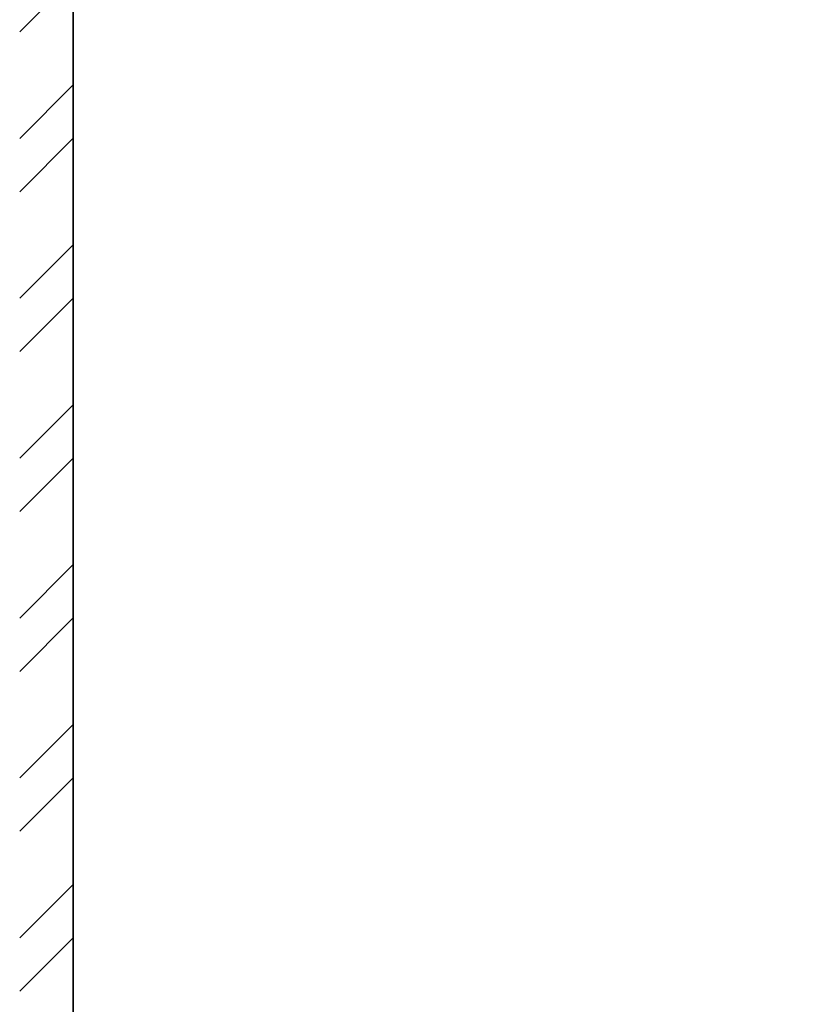
# Model space of a CAD drawing. Units: inches. Extents: x 1962 to 2771, y 1245 to 2660.
# Tile 10 of 114: x 2371 to 2439, y 1679 to 1762. Entities that reach past the tile are written whole.
import ezdxf

# ---------------------------------------------------------------- set-up
doc = ezdxf.new("R2010")
doc.units = ezdxf.units.IN
doc.layers.add('A-WALL', color=7, linetype='Continuous', lineweight=35)
doc.layers.add('A-WALL-PATT', color=252, linetype='Continuous', lineweight=13)

msp = doc.modelspace()

# ---------------------------------------------------------------- hatches: boundary and pattern name
at = {"layer": 'A-WALL-PATT'}
h = msp.add_hatch(dxfattribs=at)
h.set_pattern_fill('ANSI32', color=256)
h.paths.add_polyline_path([(2090.8074, 2467.3437), (2141.6481, 2467.3437), (2141.6481, 2469.5937), (2141.6481, 2471.8437), (2086.3074, 2471.8437), (2086.3074, 2422.5333), (2090.8074, 2422.5333)])
h.paths.add_polyline_path([(2282.7664, 2471.8437), (2204.8982, 2471.8437), (2204.8982, 2467.3437), (2234.8074, 2467.3437), (2234.8074, 2311.3437), (2228.7492, 2311.3437), (2228.7492, 2306.8437), (2234.8074, 2306.8437), (2331.9227, 2306.8437), (2331.9227, 2309.0937), (2331.9227, 2311.3437), (2239.3074, 2311.3437), (2239.3074, 2467.3437), (2282.7664, 2467.3437), (2282.7664, 2469.5937)])
h.paths.add_polyline_path([(2471.4531, 2519.8437), (2552.011, 2519.8437), (2564.3996, 2519.8437), (2564.3996, 2511.1389), (2568.8996, 2511.1389), (2568.8996, 2524.3437), (2466.9531, 2524.3437), (2466.9531, 2471.8437), (2450.0749, 2471.8437), (2446.4672, 2471.8437), (2446.4672, 2467.3437), (2450.0749, 2467.3437), (2475.9988, 2467.3437), (2475.9988, 2469.5937), (2475.9988, 2471.8437), (2471.4531, 2471.8437)])
h.paths.add_polyline_path([(2575.2231, 2469.5937), (2575.2231, 2471.8437), (2568.8996, 2471.8437), (2568.8996, 2487.1389), (2564.3996, 2487.1389), (2564.3996, 2471.8437), (2556.511, 2471.8437), (2499.2904, 2471.8437), (2499.2904, 2467.3437), (2507.8074, 2467.3437), (2507.8074, 2311.3437), (2414.863, 2311.3437), (2414.863, 2306.8437), (2512.3074, 2306.8437), (2517.0114, 2306.8437), (2517.0114, 2309.0937), (2517.0114, 2311.3437), (2512.3074, 2311.3437), (2512.3074, 2467.3437), (2575.2231, 2467.3437)])
h.paths.add_polyline_path([(2660.8074, 2471.8437), (2600.9602, 2471.8437), (2600.9602, 2467.3437), (2656.3074, 2467.3437), (2656.3074, 2432.5704), (2660.8074, 2432.5704)])
h.paths.add_polyline_path([(2660.8074, 2372.5704), (2656.3074, 2372.5704), (2656.3074, 2311.3437), (2600.276, 2311.3437), (2600.276, 2309.0937), (2600.276, 2306.8437), (2656.3074, 2306.8437), (2656.3074, 2296.2593), (2660.8074, 2296.2593)])
h.paths.add_polyline_path([(2572.3074, 2306.8437), (2577.1385, 2306.8437), (2577.1385, 2311.3437), (2551.082, 2311.3437), (2551.082, 2306.8437), (2567.8074, 2306.8437), (2567.8074, 2258.8437), (2540.0574, 2258.8437), (2540.0574, 2256.5937), (2540.0574, 2254.3437), (2567.8074, 2254.3437), (2656.3074, 2254.3437), (2656.3074, 2236.9085), (2660.8074, 2236.9085), (2660.8074, 2272.2593), (2656.3074, 2272.2593), (2656.3074, 2258.8437), (2572.3074, 2258.8437)])
h.paths.add_polyline_path([(2512.3074, 2254.3437), (2518.8716, 2254.3437), (2518.8716, 2256.5937), (2518.8716, 2258.8437), (2507.8074, 2258.8437), (2507.8074, 2177.8437), (2567.8074, 2177.8437), (2567.8074, 2172.9628), (2572.3074, 2172.9628), (2572.3074, 2177.8437), (2656.3074, 2177.8437), (2656.3074, 2166.4846), (2660.8074, 2166.4846), (2660.8074, 2200.9085), (2656.3074, 2200.9085), (2656.3074, 2182.3437), (2512.3074, 2182.3437)])
h.paths.add_polyline_path([(2656.3074, 2129.8437), (2572.3074, 2129.8437), (2572.3074, 2150.3044), (2570.0574, 2150.3044), (2567.8074, 2150.3044), (2567.8074, 2129.8437), (2507.8074, 2129.8437), (2507.8074, 2116.3027), (2510.0574, 2116.3027), (2512.3074, 2116.3027), (2512.3074, 2125.3437), (2567.8074, 2125.3437), (2572.3074, 2125.3437), (2656.3074, 2125.3437)])
h.paths.add_polyline_path([(2090.8074, 2362.5333), (2086.3074, 2362.5333), (2086.3074, 2298.6242), (2090.8074, 2298.6242), (2090.8074, 2306.8437), (2174.8074, 2306.8437), (2174.8074, 2286.4178), (2179.3074, 2286.4178), (2179.3074, 2306.8437), (2192.8641, 2306.8437), (2192.8641, 2309.0937), (2192.8641, 2311.3437), (2090.8074, 2311.3437)])
h.paths.add_polyline_path([(2209.156, 2258.8437), (2179.3074, 2258.8437), (2179.3074, 2263.2236), (2177.0574, 2263.2236), (2174.8074, 2263.2236), (2174.8074, 2258.8437), (2090.8074, 2258.8437), (2090.8074, 2274.6242), (2086.3074, 2274.6242), (2086.3074, 2238.2967), (2088.5574, 2238.2967), (2090.8074, 2238.2967), (2090.8074, 2254.3437), (2209.156, 2254.3437)])
h.paths.add_polyline_path([(2090.8074, 2177.8437), (2234.8074, 2177.8437), (2234.8074, 2173.1428), (2239.3074, 2173.1428), (2239.3074, 2258.8437), (2230.8442, 2258.8437), (2230.8442, 2256.5937), (2230.8442, 2254.3437), (2234.8074, 2254.3437), (2234.8074, 2182.3437), (2090.8074, 2182.3437), (2090.8074, 2202.2967), (2086.3074, 2202.2967), (2086.3074, 2140.0389), (2090.8074, 2140.0389)])
h.paths.add_polyline_path([(2090.8074, 2080.0389), (2086.3074, 2080.0389), (2086.3074, 2033.8437), (2090.8074, 2033.8437)], flags=17)
h.paths.add_polyline_path([(2244.9405, 2033.8437), (2239.3074, 2033.8437), (2239.3074, 2142.0665), (2237.2592, 2142.0665), (2234.8074, 2142.0665), (2234.8074, 2033.8437), (2090.8074, 2033.8437), (2076.5204, 2033.8437), (2072.0204, 2033.8437), (2072.0204, 2000.4493), (2076.5204, 2000.4493), (2076.5204, 2029.3437), (2090.8074, 2029.3437), (2244.9405, 2029.3437), (2244.9405, 2031.5937)])
h.paths.add_polyline_path([(2234.8074, 1933.3437), (2076.5204, 1933.3437), (2076.5204, 1952.4493), (2074.2704, 1952.4493), (2072.0204, 1952.4493), (2072.0204, 1933.3437), (2072.0204, 1928.8437), (2234.8074, 1928.8437)])
h.paths.add_polyline_path([(2090.8074, 1928.8437), (2086.3074, 1928.8437), (2086.3074, 1906.5013), (2090.8074, 1906.5013)])
h.paths.add_polyline_path([(2090.8074, 1846.5013), (2086.3074, 1846.5013), (2086.3074, 1769.9917), (2088.5574, 1769.9917), (2090.8074, 1769.9917), (2090.8074, 1780.3437), (2234.8074, 1780.3437), (2234.8074, 1708.3437), (2230.3764, 1708.3437), (2230.3764, 1703.8437), (2239.3074, 1703.8437), (2239.3074, 1792.6669), (2237.0574, 1792.6669), (2234.8074, 1792.6669), (2234.8074, 1784.8437), (2090.8074, 1784.8437)])
h.paths.add_polyline_path([(2239.3074, 1928.8437), (2244.9405, 1928.8437), (2244.9405, 1931.0937), (2244.9405, 1933.3437), (2234.8074, 1933.3437), (2234.8074, 1928.8437), (2234.8074, 1825.5949), (2239.3074, 1825.5949)])
h.paths.add_polyline_path([(2148.0425, 1649.0937), (2148.0425, 1651.3437), (2090.8074, 1651.3437), (2090.8074, 1646.8437), (2148.0425, 1646.8437)], flags=0)
h.paths.add_polyline_path([(2207.5601, 1708.3437), (2090.8074, 1708.3437), (2090.8074, 1703.8437), (2174.8074, 1703.8437), (2174.8074, 1651.3437), (2170.4457, 1651.3437), (2170.4457, 1646.8437), (2195.9924, 1646.8437), (2195.9924, 1649.0937), (2195.9924, 1651.3437), (2179.3074, 1651.3437), (2179.3074, 1703.8437), (2207.5601, 1703.8437), (2207.5601, 1706.0937)])
h.paths.add_polyline_path([(2090.8074, 1733.9917), (2086.3074, 1733.9917), (2086.3074, 1696.1032), (2088.5574, 1696.1032), (2090.8074, 1696.1032)])
h.paths.add_polyline_path([(2090.8074, 1672.1032), (2086.3074, 1672.1032), (2086.3074, 1600.3335), (2090.8074, 1600.3335)])
h.paths.add_polyline_path([(2090.8074, 1540.3335), (2086.3074, 1540.3335), (2086.3074, 1486.3437), (2139.6766, 1486.3437), (2139.6766, 1490.8437), (2090.8074, 1490.8437)])
h.paths.add_polyline_path([(2302.3876, 1490.8437), (2239.3074, 1490.8437), (2239.3074, 1646.8437), (2335.9994, 1646.8437), (2335.9994, 1651.3437), (2229.884, 1651.3437), (2229.884, 1646.8437), (2234.8074, 1646.8437), (2234.8074, 1490.8437), (2202.7103, 1490.8437), (2202.7103, 1488.5937), (2202.7103, 1486.3437), (2275.0699, 1486.3437), (2275.0699, 1475.772), (2279.5699, 1475.772), (2279.5699, 1486.3437), (2302.3876, 1486.3437)])
h.paths.add_polyline_path([(2279.5699, 1451.772), (2275.0699, 1451.772), (2275.0699, 1438.3437), (2174.8074, 1438.3437), (2174.8074, 1486.3437), (2179.7922, 1486.3437), (2179.7922, 1490.8437), (2163.3585, 1490.8437), (2163.3585, 1488.5937), (2163.3585, 1486.3437), (2170.3074, 1486.3437), (2170.3074, 1433.8437), (2279.5699, 1433.8437)])
h.paths.add_polyline_path([(2427.2363, 1490.8437), (2375.8074, 1490.8437), (2375.8074, 1646.8437), (2381.6401, 1646.8437), (2381.6401, 1651.3437), (2365.887, 1651.3437), (2365.887, 1649.0937), (2365.887, 1646.8437), (2371.3074, 1646.8437), (2371.3074, 1490.8437), (2327.5627, 1490.8437), (2327.5627, 1488.5937), (2327.5627, 1486.3437), (2371.3074, 1486.3437), (2371.3074, 1433.8437), (2375.8074, 1433.8437), (2375.8074, 1486.3437), (2427.2363, 1486.3437)])
h.paths.add_polyline_path([(2512.3074, 1646.8437), (2519.4351, 1646.8437), (2519.4351, 1649.0937), (2519.4351, 1651.3437), (2507.8074, 1651.3437), (2416.0063, 1651.3437), (2416.0063, 1649.0937), (2416.0063, 1646.8437), (2507.8074, 1646.8437), (2507.8074, 1490.8437), (2497.0532, 1490.8437), (2497.0532, 1488.5937), (2497.0532, 1486.3437), (2574.9344, 1486.3437), (2574.9344, 1476.0181), (2579.4344, 1476.0181), (2579.4344, 1486.3437), (2584.4872, 1486.3437), (2584.3074, 1490.8437), (2512.3074, 1490.8437)])
h.paths.add_polyline_path([(2470.5091, 1486.3437), (2473.9767, 1486.3437), (2473.9767, 1490.8437), (2449.6605, 1490.8437), (2449.6605, 1488.5937), (2449.6605, 1486.3437), (2466.0091, 1486.3437), (2466.0091, 1433.8437), (2470.5091, 1433.8437), (2579.4344, 1433.8437), (2579.4344, 1452.0181), (2574.9344, 1452.0181), (2574.9344, 1438.3437), (2554.5091, 1438.3437), (2470.5091, 1438.3437)])
h.paths.add_polyline_path([(2656.3074, 1490.8437), (2611.86, 1490.8437), (2611.86, 1486.3437), (2656.3074, 1486.3437)])
h.paths.add_polyline_path([(2660.8074, 1532.7007), (2658.5574, 1532.7007), (2656.3074, 1532.7007), (2656.3074, 1486.3437), (2660.8074, 1486.3437)])
h.paths.add_polyline_path([(2660.8074, 1664.9663), (2656.3074, 1664.9663), (2656.3074, 1651.3437), (2602.2313, 1651.3437), (2602.2313, 1646.8437), (2656.3074, 1646.8437), (2656.3074, 1592.7007), (2660.8074, 1592.7007)])
h.paths.add_polyline_path([(2660.8074, 1724.5221), (2656.3074, 1724.5221), (2656.3074, 1703.8437), (2542.4725, 1703.8437), (2542.4725, 1699.3437), (2567.8074, 1699.3437), (2567.8074, 1651.3437), (2552.7766, 1651.3437), (2552.7766, 1649.0937), (2552.7766, 1646.8437), (2577.2878, 1646.8437), (2577.2878, 1649.0937), (2577.2878, 1651.3437), (2572.3074, 1651.3437), (2572.3074, 1699.3437), (2656.3074, 1699.3437), (2656.3074, 1688.9663), (2660.8074, 1688.9663)])
h.paths.add_polyline_path([(2660.8074, 1880.6524), (2656.3074, 1880.6524), (2656.3074, 1832.8437), (2512.3074, 1832.8437), (2512.3074, 1837.8959), (2507.8074, 1837.8959), (2507.8074, 1828.3437), (2567.8074, 1828.3437), (2567.8074, 1804.3437), (2572.3074, 1804.3437), (2572.3074, 1828.3437), (2656.3074, 1828.3437), (2656.3074, 1818.6778), (2660.8074, 1818.6778)])
h.paths.add_polyline_path([(2660.8074, 1794.6778), (2656.3074, 1794.6778), (2656.3074, 1780.3437), (2572.3074, 1780.3437), (2572.3074, 1783.0303), (2570.0574, 1783.0303), (2567.8074, 1783.0303), (2567.8074, 1780.3437), (2507.8074, 1780.3437), (2507.8074, 1699.3437), (2517.8858, 1699.3437), (2517.8858, 1701.5937), (2517.8858, 1703.8437), (2512.3074, 1703.8437), (2512.3074, 1775.8437), (2656.3074, 1775.8437), (2656.3074, 1760.5221), (2660.8074, 1760.5221)])
h.paths.add_polyline_path([(2660.8074, 1981.3437), (2660.8074, 2020.2808), (2658.5574, 2020.2808), (2656.3074, 2020.2808), (2656.3074, 1981.3437), (2512.3074, 1981.3437), (2512.3074, 2086.6996), (2507.8074, 2086.6996), (2507.8074, 1981.3437), (2375.8074, 1981.3437), (2375.8074, 1986.8505), (2373.5574, 1986.8505), (2371.3074, 1986.8505), (2371.3074, 1973.2607), (2375.8074, 1973.2607), (2375.8074, 1976.8437), (2507.8074, 1976.8437), (2507.8074, 1865.4281), (2510.0574, 1865.4281), (2512.3074, 1865.4281), (2512.3074, 1976.8437), (2660.8074, 1976.8437)])
h.paths.add_polyline_path([(2375.8074, 1940.297), (2373.5574, 1940.297), (2371.3074, 1940.297), (2371.3074, 1933.3437), (2278.4434, 1933.3437), (2278.4434, 1928.8437), (2371.3074, 1928.8437), (2371.3074, 1651.3437), (2375.8074, 1651.3437)])
h.paths.add_polyline_path([(2660.8074, 1976.8437), (2656.3074, 1976.8437), (2656.3074, 1940.6524), (2660.8074, 1940.6524)], flags=17)
h.paths.add_polyline_path([(2660.8074, 2142.4846), (2656.3074, 2142.4846), (2656.3074, 2080.2808), (2660.8074, 2080.2808)])
h.paths.add_polyline_path([(2381.4189, 2311.3437), (2375.8074, 2311.3437), (2375.8074, 2467.3437), (2424.7242, 2467.3437), (2424.7242, 2469.5937), (2424.7242, 2471.8437), (2375.8074, 2471.8437), (2375.8074, 2524.3437), (2371.3074, 2524.3437), (2371.3074, 2471.8437), (2307.2097, 2471.8437), (2307.2097, 2467.3437), (2371.3074, 2467.3437), (2371.3074, 2311.3437), (2366.8901, 2311.3437), (2366.8901, 2306.8437), (2371.3074, 2306.8437), (2371.3074, 2033.8437), (2279.6589, 2033.8437), (2279.6589, 2029.3437), (2371.3074, 2029.3437), (2371.3074, 2014.2598), (2375.8074, 2014.2598), (2375.8074, 2306.8437), (2381.4189, 2306.8437)])
h.paths.add_polyline_path([(2263.3074, 2524.3437), (2170.3074, 2524.3437), (2170.3074, 2519.8437), (2170.3074, 2471.8437), (2165.0312, 2471.8437), (2165.0312, 2467.3437), (2179.6721, 2467.3437), (2179.6721, 2469.5161), (2179.6721, 2471.8437), (2174.8074, 2471.8437), (2174.8074, 2519.8437), (2258.8074, 2519.8437), (2258.8074, 2511.6436), (2263.3074, 2511.6436)])
h.paths.add_polyline_path([(2245.0232, 1361.4123), (2492.9468, 1361.4123), (2492.9468, 1398.505), (2245.0232, 1398.505)], flags=9)
h.paths.add_polyline_path([(2388.1434, 2086.6936), (2425.0704, 2086.6936), (2425.0704, 2105.3509), (2388.1434, 2105.3509)], flags=9)
h.paths.add_polyline_path([(2404.922, 2242.6744), (2445.7337, 2242.6744), (2445.7337, 2261.3318), (2404.922, 2261.3318)], flags=9)
h.paths.add_polyline_path([(2269.4107, 2156.7935), (2306.3378, 2156.7935), (2306.3378, 2175.4508), (2269.4107, 2175.4508)], flags=9)
h.paths.add_polyline_path([(2269.3277, 2233.4343), (2306.2547, 2233.4343), (2306.2547, 2252.0917), (2269.3277, 2252.0917)], flags=9)
h.paths.add_polyline_path([(2431.6052, 2320.6922), (2470.4456, 2320.6922), (2470.4456, 2339.3495), (2431.6052, 2339.3495)], flags=25)
h.paths.add_polyline_path([(2249.6902, 2315.7608), (2288.5306, 2315.7608), (2288.5306, 2334.4182), (2249.6902, 2334.4182)], flags=25)
h.paths.add_polyline_path([(2096.9301, 2314.3181), (2135.7704, 2314.3181), (2135.7704, 2332.9755), (2096.9301, 2332.9755)], flags=25)
h.paths.add_polyline_path([(2134.3475, 2285.7089), (2161.4655, 2285.7089), (2161.4655, 2304.3662), (2134.3475, 2304.3662)], flags=9)
h.paths.add_polyline_path([(2126.5155, 2209.4076), (2159.9227, 2209.4076), (2159.9227, 2228.065), (2126.5155, 2228.065)], flags=25)
h.paths.add_polyline_path([(2110.5753, 2141.5299), (2149.4157, 2141.5299), (2149.4157, 2160.1872), (2110.5753, 2160.1872)], flags=25)
h.paths.add_polyline_path([(2249.8618, 1968.3317), (2286.3966, 1968.3317), (2286.3966, 1986.989), (2249.8618, 1986.989)], flags=9)
h.paths.add_polyline_path([(2395.9507, 1777.0051), (2436.7624, 1777.0051), (2436.7624, 1795.6625), (2395.9507, 1795.6625)], flags=9)
h.paths.add_polyline_path([(2398.5259, 1888.5651), (2435.0062, 1888.5651), (2435.0062, 1907.2224), (2398.5259, 1907.2224)], flags=25)
h.paths.add_polyline_path([(2259.3506, 1728.3559), (2296.2776, 1728.3559), (2296.2776, 1747.0132), (2259.3506, 1747.0132)], flags=9)
h.paths.add_polyline_path([(2271.3698, 1845.268), (2308.2968, 1845.268), (2308.2968, 1863.9253), (2271.3698, 1863.9253)], flags=9)
h.paths.add_polyline_path([(2120.9355, 1786.3027), (2159.7759, 1786.3027), (2159.7759, 1804.9601), (2120.9355, 1804.9601)], flags=25)
h.paths.add_polyline_path([(2121.3164, 1732.1043), (2154.7236, 1732.1043), (2154.7236, 1750.7616), (2121.3164, 1750.7616)], flags=25)
h.paths.add_polyline_path([(2118.3706, 1678.8997), (2147.5282, 1678.8997), (2147.5282, 1697.557), (2118.3706, 1697.557)], flags=25)
h.paths.add_polyline_path([(2385.9227, 1493.557), (2424.763, 1493.557), (2424.763, 1512.2143), (2385.9227, 1512.2143)], flags=25)
h.paths.add_polyline_path([(2248.7058, 1500.0256), (2287.5462, 1500.0256), (2287.5462, 1518.6829), (2248.7058, 1518.6829)], flags=25)
h.paths.add_polyline_path([(2104.1669, 1617.3771), (2143.0073, 1617.3771), (2143.0073, 1636.0344), (2104.1669, 1636.0344)], flags=9)
h.paths.add_polyline_path([(2096.0714, 1447.8824), (2137.3845, 1447.8824), (2137.3845, 1458.1859), (2096.0714, 1458.1859)], flags=9)
h.paths.add_polyline_path([(2180.6114, 1440.325), (2209.7689, 1440.325), (2209.7689, 1458.9823), (2180.6114, 1458.9823)], flags=25)
h.paths.add_polyline_path([(2316.1698, 1447.9637), (2357.4829, 1447.9637), (2357.4829, 1458.2673), (2316.1698, 1458.2673)], flags=9)
h.paths.add_polyline_path([(2397.6187, 1447.9637), (2438.9318, 1447.9637), (2438.9318, 1458.2673), (2397.6187, 1458.2673)], flags=9)
h.paths.add_polyline_path([(2473.0778, 1439.5953), (2502.2354, 1439.5953), (2502.2354, 1458.2527), (2473.0778, 1458.2527)], flags=25)
h.paths.add_polyline_path([(2589.7027, 1447.8819), (2631.0158, 1447.8819), (2631.0158, 1458.1855), (2589.7027, 1458.1855)], flags=9)
h.paths.add_polyline_path([(2522.4009, 1497.5285), (2561.2413, 1497.5285), (2561.2413, 1516.1859), (2522.4009, 1516.1859)], flags=25)
h.paths.add_polyline_path([(2579.6565, 1671.3482), (2608.8141, 1671.3482), (2608.8141, 1690.0056), (2579.6565, 1690.0056)], flags=25)
h.paths.add_polyline_path([(2544.7038, 1725.5064), (2578.1111, 1725.5064), (2578.1111, 1744.1637), (2544.7038, 1744.1637)], flags=25)
h.paths.add_polyline_path([(2578.1191, 1807.472), (2607.2766, 1807.472), (2607.2766, 1826.1293), (2578.1191, 1826.1293)], flags=25)
h.paths.add_polyline_path([(2595.0614, 1835.1839), (2633.9018, 1835.1839), (2633.9018, 1853.8413), (2595.0614, 1853.8413)], flags=25)
h.paths.add_polyline_path([(2567.0097, 2097.7035), (2605.8501, 2097.7035), (2605.8501, 2116.3609), (2567.0097, 2116.3609)], flags=9)
h.paths.add_polyline_path([(2586.644, 2134.6454), (2615.8015, 2134.6454), (2615.8015, 2153.3027), (2586.644, 2153.3027)], flags=9)
h.paths.add_polyline_path([(2544.6185, 2212.6783), (2578.0258, 2212.6783), (2578.0258, 2231.3356), (2544.6185, 2231.3356)], flags=25)
h.paths.add_polyline_path([(2577.0273, 2256.9023), (2606.1849, 2256.9023), (2606.1849, 2275.5597), (2577.0273, 2275.5597)], flags=24)
h.paths.add_polyline_path([(2605.2683, 2315.2821), (2644.1087, 2315.2821), (2644.1087, 2333.9395), (2605.2683, 2333.9395)], flags=25)
h.paths.add_polyline_path([(2583.1244, 2496.1815), (2624.4375, 2496.1815), (2624.4375, 2506.4851), (2583.1244, 2506.4851)], flags=9)
h.paths.add_polyline_path([(2474.761, 2497.0823), (2503.9185, 2497.0823), (2503.9185, 2515.7397), (2474.761, 2515.7397)], flags=25)
h.paths.add_polyline_path([(2387.5787, 2494.2563), (2428.902, 2494.2563), (2428.902, 2504.5598), (2387.5787, 2504.5598)], flags=9)
h.paths.add_polyline_path([(2300.1657, 2500.1564), (2341.4788, 2500.1564), (2341.4788, 2510.46), (2300.1657, 2510.46)], flags=25)
h.paths.add_polyline_path([(2176.8589, 2497.5843), (2206.0165, 2497.5843), (2206.0165, 2516.2416), (2176.8589, 2516.2416)], flags=25)
h.paths.add_polyline_path([(2097.4668, 2494.9762), (2138.7799, 2494.9762), (2138.7799, 2505.2798), (2097.4668, 2505.2798)], flags=9)

# ---------------------------------------------------------------- linework, layer by layer
at = {"layer": 'A-WALL'}
msp.add_line((2375.8074, 1941.894), (2375.8074, 1651.3437), dxfattribs=at)

doc.saveas('drawing.dxf')
